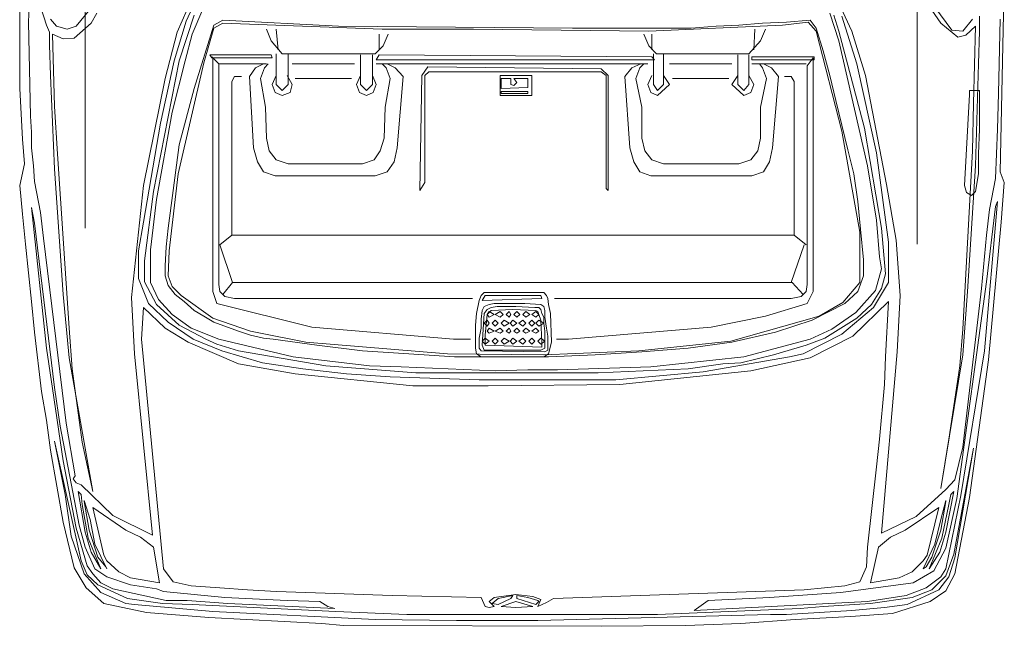
# Model space of a CAD drawing. Units: inches. Extents: x -9 to 646, y -802 to 47.
# Tile 4 of 17: x 432 to 486, y -666 to -633. Entities that reach past the tile are written whole.
import ezdxf

# ---------------------------------------------------------------- set-up
doc = ezdxf.new("R2010")
doc.units = ezdxf.units.IN
doc.header["$MEASUREMENT"] = 0
doc.layers.add('A-SITE-VEHI', color=8, linetype='Continuous', lineweight=9)

msp = doc.modelspace()

# ---------------------------------------------------------------- linework, layer by layer
at = {"layer": 'A-SITE-VEHI'}
for p, q in [((435.913, -624.106), (435.913, -643.944)), ((481.443, -624.866), (481.443, -644.812)), ((432.336, -626.818), (432.336, -636.303)), ((432.933, -629.311), (432.824, -632.671)), ((485.995, -640.855), (486.213, -630.124)), ((433.799, -632.833), (433.311, -631.316)), ((440.953, -633.212), (441.93, -630.99)), ((442.092, -631.207), (441.442, -632.617)), ((477.864, -633.159), (476.836, -630.936)), ((436.184, -631.967), (435.425, -632.888)), ((442.363, -631.967), (441.766, -633.321)), ((483.339, -633.104), (482.418, -631.858)), ((434.341, -632.888), (434.017, -632.509)), ((436.564, -632.182), (436.239, -632.726)), ((441.875, -632.291), (441.062, -634.785)), ((477.16, -633.701), (476.672, -632.182)), ((477.16, -633.159), (476.889, -632.291)), ((478.137, -634.947), (477.322, -632.346)), ((482.256, -632.02), (482.742, -632.726)), ((484.479, -632.509), (483.935, -633.159)), ((484.856, -633.159), (484.856, -632.346)), ((485.995, -632.509), (485.886, -636.574)), ((432.824, -632.671), (432.933, -637.82)), ((433.961, -633.212), (433.799, -632.833)), ((434.938, -633.05), (434.341, -632.888)), ((435.425, -632.888), (434.938, -633.05)), ((436.239, -632.726), (435.318, -633.539)), ((441.442, -632.617), (440.791, -634.785)), ((442.958, -632.833), (441.875, -636.303)), ((442.958, -632.997), (442.417, -634.893)), ((443.447, -632.562), (442.958, -632.833)), ((443.447, -632.726), (442.958, -632.997)), ((449.789, -632.888), (443.447, -632.562)), ((452.173, -633.05), (443.447, -632.726)), ((445.832, -633.05), (446.103, -633.701)), ((446.374, -633.05), (446.482, -634.189)), ((462.581, -632.997), (449.789, -632.888)), ((457.16, -633.05), (452.173, -633.05)), ((466.753, -633.159), (457.16, -633.05)), ((469.084, -632.997), (462.581, -632.997)), ((474.071, -632.833), (466.753, -633.159)), ((470.439, -632.888), (469.084, -632.997)), ((471.687, -632.833), (470.439, -632.888)), ((472.988, -632.726), (471.687, -632.833)), ((472.553, -633.05), (472.499, -634.189)), ((473.15, -633.05), (472.879, -633.701)), ((474.287, -632.671), (472.988, -632.726)), ((475.479, -632.671), (474.071, -632.833)), ((475.588, -632.562), (474.287, -632.671)), ((475.914, -633.159), (475.479, -632.671)), ((475.914, -632.997), (475.588, -632.562)), ((476.294, -634.243), (475.914, -632.997)), ((482.742, -632.726), (483.664, -633.483)), ((484.099, -633.377), (484.641, -632.888)), ((484.641, -632.888), (484.532, -637.116)), ((433.961, -633.919), (433.961, -633.212)), ((434.721, -633.592), (434.125, -633.321)), ((434.125, -633.321), (434.232, -637.278)), ((435.318, -633.539), (434.721, -633.592)), ((440.303, -635.761), (440.953, -633.212)), ((441.766, -633.321), (441.389, -634.785)), ((452.011, -633.321), (452.011, -634.189)), ((452.229, -633.972), (452.5, -633.321)), ((466.753, -633.972), (466.482, -633.321)), ((466.917, -633.321), (466.917, -634.189)), ((477.322, -638.633), (475.914, -633.159)), ((478.57, -638.47), (477.16, -633.159)), ((478.623, -635.597), (477.864, -633.159)), ((483.935, -633.159), (483.339, -633.104)), ((483.664, -633.483), (484.099, -633.377)), ((484.803, -634.947), (484.856, -633.159)), ((434.017, -635.597), (433.961, -633.919)), ((446.103, -633.701), (446.7, -634.405)), ((451.794, -634.405), (452.229, -633.972)), ((467.188, -634.405), (466.753, -633.972)), ((472.879, -633.701), (472.228, -634.405)), ((478.732, -640.531), (477.16, -633.701)), ((446.103, -634.46), (442.743, -634.46)), ((442.743, -634.46), (442.852, -634.622)), ((442.852, -634.569), (443.232, -634.947)), ((442.852, -634.622), (446.158, -634.622)), ((442.905, -634.622), (442.905, -647.414)), ((446.158, -634.622), (446.103, -634.46)), ((446.374, -636.086), (446.374, -634.405)), ((446.7, -634.405), (451.794, -634.405)), ((447.024, -634.405), (447.024, -636.086)), ((450.981, -636.086), (450.981, -634.46)), ((451.632, -634.46), (451.632, -636.086)), ((452.011, -634.46), (451.849, -634.731)), ((466.917, -634.569), (452.011, -634.46)), ((467.079, -634.731), (466.917, -634.569)), ((467.024, -636.086), (467.024, -634.405)), ((472.228, -634.405), (467.188, -634.405)), ((467.568, -634.405), (467.568, -636.086)), ((471.631, -636.086), (471.631, -634.46)), ((472.228, -634.46), (472.228, -636.086)), ((475.806, -634.569), (472.39, -634.569)), ((472.39, -634.569), (472.39, -634.731)), ((475.752, -634.622), (475.426, -635.055)), ((475.752, -634.622), (475.752, -647.414)), ((475.806, -634.731), (475.806, -634.569)), ((476.672, -635.597), (476.294, -634.243)), ((441.062, -634.785), (439.652, -641.939)), ((440.791, -634.785), (440.032, -638.2)), ((441.389, -634.785), (440.683, -637.602)), ((442.417, -634.893), (441.009, -640.964)), ((445.832, -634.947), (443.232, -634.947)), ((443.232, -634.947), (443.232, -647.035)), ((444.91, -635.653), (445.237, -635.164)), ((445.237, -635.164), (445.67, -634.947)), ((445.507, -635.761), (445.723, -635.164)), ((445.723, -635.164), (445.941, -634.947)), ((450.657, -634.947), (447.242, -634.947)), ((451.849, -634.731), (467.079, -634.731)), ((466.699, -634.947), (451.849, -634.947)), ((452.173, -634.947), (452.391, -635.164)), ((452.391, -635.164), (452.606, -635.761)), ((452.444, -634.947), (452.877, -635.164)), ((452.877, -635.164), (453.312, -635.653)), ((454.667, -635.111), (454.343, -635.597)), ((464.153, -635.218), (454.667, -635.111)), ((465.454, -635.653), (465.831, -635.164)), ((465.831, -635.164), (466.32, -634.947)), ((466.049, -635.761), (466.266, -635.164)), ((466.266, -635.164), (466.482, -634.947)), ((471.307, -634.947), (467.892, -634.947)), ((472.39, -634.731), (475.806, -634.731)), ((475.372, -634.947), (472.39, -634.947)), ((472.823, -634.947), (472.988, -635.164)), ((472.988, -635.164), (473.203, -635.761)), ((473.041, -634.947), (473.474, -635.164)), ((473.474, -635.164), (473.854, -635.653)), ((475.426, -635.055), (475.426, -647.035)), ((479.221, -639.825), (478.137, -634.947)), ((484.641, -640.531), (484.803, -634.947)), ((434.232, -640.693), (434.017, -635.597)), ((444.098, -635.653), (443.935, -635.924)), ((444.477, -635.653), (444.098, -635.653)), ((445.128, -639.554), (444.91, -635.653)), ((446.158, -636.086), (446.374, -635.597)), ((446.971, -635.597), (447.242, -636.086)), ((450.763, -636.086), (450.981, -635.597)), ((451.632, -635.597), (451.849, -636.086)), ((453.312, -635.653), (452.986, -639.554)), ((454.343, -635.597), (454.234, -641.886)), ((454.505, -635.597), (454.72, -635.382)), ((454.505, -641.452), (454.505, -635.597)), ((454.72, -635.382), (464.153, -635.382)), ((460.358, -635.597), (458.624, -635.597)), ((458.624, -635.597), (458.624, -636.683)), ((460.358, -636.683), (460.358, -635.597)), ((464.532, -635.597), (464.153, -635.218)), ((464.153, -635.382), (464.423, -635.597)), ((464.423, -635.597), (464.423, -641.777)), ((464.532, -641.886), (464.532, -635.597)), ((465.725, -639.554), (465.454, -635.653)), ((466.699, -636.086), (466.917, -635.597)), ((467.568, -635.597), (467.892, -636.086)), ((471.307, -636.086), (471.631, -635.597)), ((472.228, -635.597), (472.499, -636.086)), ((473.854, -635.653), (473.53, -639.554)), ((474.18, -635.653), (474.558, -635.653)), ((474.558, -635.653), (474.722, -635.924)), ((476.998, -636.954), (476.672, -635.597)), ((479.762, -641.559), (478.623, -635.597)), ((439.11, -641.615), (440.303, -635.761)), ((443.935, -635.924), (443.935, -644.324)), ((445.778, -637.331), (445.507, -635.761)), ((446.32, -636.519), (446.158, -636.086)), ((446.7, -636.41), (446.374, -636.086)), ((447.024, -636.086), (446.7, -636.41)), ((447.242, -636.086), (447.133, -636.519)), ((447.404, -635.761), (450.492, -635.761)), ((450.928, -636.519), (450.763, -636.086)), ((451.307, -636.41), (450.981, -636.086)), ((451.632, -636.086), (451.307, -636.41)), ((451.849, -636.086), (451.685, -636.519)), ((452.606, -635.761), (452.335, -637.331)), ((459.219, -635.761), (458.677, -635.761)), ((458.677, -635.761), (458.677, -636.303)), ((458.677, -636.303), (460.14, -636.248)), ((459.219, -636.086), (459.219, -635.761)), ((459.383, -636.139), (459.219, -636.086)), ((460.14, -635.761), (459.383, -635.761)), ((459.383, -635.761), (459.545, -635.977)), ((459.545, -635.977), (459.383, -636.139)), ((460.14, -636.248), (460.14, -635.761)), ((466.375, -637.331), (466.049, -635.761)), ((466.862, -636.519), (466.699, -636.086)), ((467.241, -636.41), (467.024, -636.086)), ((467.892, -636.086), (467.241, -636.683)), ((467.568, -636.086), (467.241, -636.41)), ((468.054, -635.761), (471.145, -635.761)), ((471.957, -636.683), (471.307, -636.086)), ((471.957, -636.41), (471.631, -636.086)), ((472.228, -636.086), (471.957, -636.41)), ((472.499, -636.086), (472.337, -636.519)), ((473.203, -635.761), (472.879, -637.331)), ((474.722, -635.924), (474.722, -644.324)), ((432.336, -636.303), (432.498, -639.068)), ((441.875, -636.303), (441.062, -639.392)), ((446.7, -636.683), (446.32, -636.519)), ((447.133, -636.519), (446.7, -636.683)), ((451.307, -636.683), (450.928, -636.519)), ((451.685, -636.519), (451.307, -636.683)), ((458.624, -636.683), (460.358, -636.683)), ((460.14, -636.465), (458.677, -636.465)), ((458.677, -636.465), (458.677, -636.574)), ((458.677, -636.574), (460.14, -636.574)), ((460.14, -636.574), (460.14, -636.465)), ((467.241, -636.683), (466.862, -636.519)), ((472.337, -636.519), (471.957, -636.683)), ((484.314, -636.628), (484.043, -641.615)), ((484.856, -636.41), (484.314, -636.41)), ((484.314, -636.41), (484.314, -636.628)), ((484.856, -638.524), (484.856, -636.41)), ((485.886, -636.574), (485.833, -638.524)), ((434.232, -637.278), (434.396, -639.88)), ((445.832, -639.012), (445.778, -637.331)), ((452.335, -637.331), (452.282, -639.012)), ((466.375, -639.012), (466.375, -637.331)), ((472.879, -637.331), (472.879, -639.012)), ((477.322, -638.308), (476.998, -636.954)), ((484.532, -637.116), (484.479, -639.716)), ((432.933, -637.82), (432.986, -638.688)), ((440.683, -637.602), (439.816, -642.374)), ((440.032, -638.2), (439.11, -643.62)), ((477.648, -639.663), (477.322, -638.308)), ((432.986, -638.688), (432.986, -639.554)), ((478.299, -644.161), (477.322, -638.633)), ((479.491, -643.944), (478.57, -638.47)), ((484.803, -639.88), (484.856, -638.524)), ((485.833, -638.524), (485.724, -641.235)), ((432.498, -639.068), (432.607, -640.422)), ((441.062, -639.392), (440.738, -641.886)), ((445.994, -639.716), (445.832, -639.012)), ((452.282, -639.012), (452.065, -639.716)), ((466.537, -639.716), (466.375, -639.012)), ((472.879, -639.012), (472.717, -639.716)), ((432.986, -639.554), (433.095, -640.531)), ((434.396, -639.88), (435.047, -649.419)), ((445.343, -640.313), (445.128, -639.554)), ((446.374, -640.205), (445.994, -639.716)), ((452.065, -639.716), (451.74, -640.205)), ((452.986, -639.554), (452.824, -640.313)), ((465.94, -640.313), (465.725, -639.554)), ((466.917, -640.205), (466.537, -639.716)), ((472.717, -639.716), (472.337, -640.205)), ((473.53, -639.554), (473.365, -640.313)), ((477.973, -640.964), (477.648, -639.663)), ((479.871, -644.703), (479.221, -639.825)), ((484.479, -639.716), (483.935, -649.473)), ((484.803, -640.964), (484.803, -639.88)), ((432.607, -640.422), (432.336, -641.615)), ((433.095, -640.531), (433.149, -641.397)), ((445.67, -640.855), (445.343, -640.313)), ((447.024, -640.422), (446.374, -640.205)), ((451.09, -640.422), (447.024, -640.422)), ((451.74, -640.205), (451.09, -640.422)), ((452.824, -640.313), (452.444, -640.855)), ((466.266, -640.855), (465.94, -640.313)), ((467.568, -640.422), (466.917, -640.205)), ((471.687, -640.422), (467.568, -640.422)), ((472.337, -640.205), (471.687, -640.422)), ((473.365, -640.313), (473.041, -640.855)), ((479.221, -643.511), (478.732, -640.531)), ((484.206, -647.414), (484.641, -640.531)), ((434.721, -647.577), (434.232, -640.693)), ((441.009, -640.964), (440.52, -645.192)), ((446.32, -641.073), (445.67, -640.855)), ((451.794, -641.073), (446.32, -641.073)), ((452.444, -640.855), (451.794, -641.073)), ((466.862, -641.073), (466.266, -640.855)), ((472.39, -641.073), (466.862, -641.073)), ((473.041, -640.855), (472.39, -641.073)), ((478.19, -642.481), (477.973, -640.964)), ((484.641, -641.939), (484.803, -640.964)), ((486.213, -641.452), (485.995, -640.855)), ((432.336, -641.615), (432.498, -643.187)), ((433.149, -641.397), (433.475, -643.078)), ((438.46, -647.739), (439.11, -641.615)), ((454.234, -641.886), (454.505, -641.452)), ((480.304, -644.594), (479.762, -641.559)), ((484.043, -641.615), (484.152, -641.994)), ((485.724, -641.235), (485.398, -642.916)), ((486.048, -643.62), (486.213, -641.452)), ((439.652, -641.939), (439.166, -645.734)), ((440.738, -641.886), (440.467, -643.944)), ((464.423, -641.777), (464.532, -641.886)), ((484.152, -641.994), (484.423, -642.156)), ((484.423, -642.156), (484.641, -641.939)), ((439.816, -642.374), (439.49, -645.136)), ((478.352, -643.999), (478.19, -642.481)), ((485.127, -650.665), (485.833, -642.481)), ((485.833, -642.481), (485.724, -642.752)), ((432.498, -643.187), (432.662, -644.812)), ((433.149, -643.673), (432.986, -642.807)), ((432.986, -642.807), (433.799, -650.503)), ((433.475, -643.078), (433.637, -644.488)), ((485.724, -642.752), (485.236, -646.873)), ((485.398, -642.916), (485.236, -644.324)), ((434.232, -652.67), (433.149, -643.673)), ((439.11, -643.62), (438.84, -645.192)), ((479.383, -645.516), (479.221, -643.511)), ((485.345, -651.154), (486.048, -643.62)), ((440.467, -643.944), (440.358, -644.974)), ((443.935, -644.324), (443.285, -644.865)), ((474.722, -644.324), (443.935, -644.324)), ((474.722, -644.324), (475.372, -644.865)), ((478.299, -646.926), (478.299, -644.161)), ((478.514, -645.68), (478.352, -643.999)), ((479.707, -646.437), (479.491, -643.944)), ((485.236, -644.324), (484.965, -647.25)), ((432.662, -644.812), (432.986, -647.956)), ((433.637, -644.488), (434.883, -654.622)), ((443.285, -644.865), (443.989, -646.926)), ((475.264, -644.865), (474.558, -646.926)), ((479.871, -646.926), (479.871, -644.703)), ((480.522, -647.63), (480.304, -644.594)), ((438.84, -645.192), (438.84, -646.708)), ((439.49, -645.136), (439.49, -646.926)), ((440.358, -644.974), (440.303, -646.004)), ((440.52, -645.192), (440.467, -646.546)), ((439.166, -645.734), (439.166, -646.873)), ((478.514, -646.546), (478.514, -645.68)), ((479.491, -646.167), (479.383, -645.516)), ((440.303, -646.004), (440.303, -646.546)), ((479.165, -647.359), (479.491, -646.167)), ((479.491, -647.25), (479.707, -646.437)), ((438.84, -646.708), (439.381, -648.065)), ((439.166, -646.873), (439.816, -648.118)), ((439.49, -646.926), (439.923, -647.847)), ((440.303, -646.546), (440.467, -647.088)), ((440.467, -646.546), (440.683, -647.144)), ((443.232, -647.035), (443.285, -647.414)), ((443.989, -646.926), (443.447, -647.577)), ((474.613, -646.926), (443.989, -646.926)), ((475.208, -647.577), (474.613, -646.926)), ((475.426, -647.035), (475.372, -647.414)), ((477.378, -648.01), (478.299, -646.926)), ((478.19, -647.414), (478.514, -646.546)), ((479.058, -648.28), (479.871, -646.926)), ((485.236, -646.873), (483.61, -658.741)), ((435.047, -651.045), (434.721, -647.577)), ((440.467, -647.088), (440.845, -647.577)), ((440.683, -647.144), (441.171, -647.63)), ((440.845, -647.577), (441.333, -647.956)), ((442.905, -647.414), (443.123, -648.065)), ((443.285, -647.414), (443.556, -647.685)), ((457.756, -647.468), (457.593, -647.63)), ((461.008, -647.468), (457.756, -647.468)), ((461.171, -647.63), (461.008, -647.468)), ((475.372, -647.414), (475.102, -647.685)), ((475.752, -647.414), (475.426, -648.065)), ((477.486, -648.065), (478.19, -647.414)), ((478.081, -648.551), (479.165, -647.359)), ((478.95, -648.118), (479.491, -647.25)), ((484.965, -647.25), (483.935, -655.923)), ((483.935, -650.883), (484.206, -647.414)), ((432.986, -647.956), (433.149, -649.637)), ((438.624, -650.829), (438.46, -647.739)), ((439.381, -648.065), (440.467, -649.093)), ((439.816, -648.118), (441.062, -649.257)), ((439.923, -647.847), (440.683, -648.66)), ((441.171, -647.63), (442.905, -648.878)), ((441.333, -647.956), (441.875, -648.443)), ((443.123, -648.065), (448.325, -649.364)), ((443.556, -647.685), (444.098, -647.794)), ((444.098, -647.794), (457.105, -647.794)), ((457.485, -647.901), (457.323, -648.607)), ((457.593, -647.63), (457.485, -647.901)), ((457.811, -647.63), (457.649, -647.901)), ((457.649, -647.901), (460.9, -647.794)), ((458.026, -648.118), (457.756, -648.227)), ((460.846, -647.63), (457.811, -647.63)), ((458.297, -648.065), (458.026, -648.118)), ((459.978, -648.065), (458.297, -648.065)), ((460.846, -648.118), (459.978, -648.065)), ((460.9, -647.794), (460.846, -647.63)), ((461.008, -648.227), (460.846, -648.118)), ((461.226, -647.794), (461.171, -647.63)), ((461.279, -648.118), (461.226, -647.794)), ((461.388, -648.607), (461.279, -648.118)), ((474.558, -647.794), (461.604, -647.794)), ((475.426, -648.065), (473.15, -648.769)), ((475.102, -647.685), (474.558, -647.794)), ((475.697, -648.986), (477.486, -648.065)), ((476.076, -648.769), (477.378, -648.01)), ((479.871, -647.956), (477.919, -649.852)), ((478.137, -648.878), (478.95, -648.118)), ((479.707, -650.992), (479.871, -647.956)), ((480.357, -650.721), (480.522, -647.63)), ((439.11, -648.28), (439.004, -650.015)), ((440.303, -649.419), (439.11, -648.28)), ((440.683, -648.66), (441.713, -649.419)), ((441.875, -648.443), (442.417, -648.769)), ((457.323, -648.607), (457.269, -649.257)), ((457.649, -648.443), (457.593, -648.931)), ((457.756, -648.227), (457.649, -648.443)), ((457.756, -648.607), (457.649, -650.341)), ((457.92, -648.389), (457.756, -648.607)), ((457.92, -648.66), (457.811, -649.799)), ((458.135, -648.28), (457.92, -648.389)), ((458.135, -648.443), (457.92, -648.66)), ((457.92, -648.66), (458.026, -648.498)), ((458.026, -648.822), (457.92, -648.66)), ((458.026, -648.498), (458.297, -648.66)), ((458.297, -648.66), (458.026, -648.822)), ((458.462, -648.227), (458.135, -648.28)), ((459.328, -648.389), (458.135, -648.443)), ((458.353, -648.66), (458.624, -648.498)), ((458.624, -648.822), (458.353, -648.66)), ((459.492, -648.227), (458.462, -648.227)), ((458.624, -648.498), (458.786, -648.66)), ((458.786, -648.66), (458.624, -648.822)), ((458.948, -648.66), (459.112, -648.498)), ((459.112, -648.822), (458.948, -648.66)), ((459.112, -648.498), (459.219, -648.66)), ((459.219, -648.66), (459.112, -648.822)), ((460.575, -648.443), (459.328, -648.389)), ((459.383, -648.66), (459.545, -648.498)), ((459.545, -648.822), (459.383, -648.66)), ((460.52, -648.28), (459.492, -648.227)), ((459.545, -648.498), (459.707, -648.66)), ((459.707, -648.66), (459.545, -648.822)), ((459.869, -648.66), (460.034, -648.498)), ((460.034, -648.822), (459.869, -648.66)), ((460.034, -648.498), (460.249, -648.66)), ((460.249, -648.66), (460.034, -648.822)), ((460.358, -648.66), (460.575, -648.498)), ((460.575, -648.822), (460.358, -648.66)), ((460.738, -648.28), (460.52, -648.28)), ((460.684, -648.498), (460.575, -648.443)), ((460.575, -648.498), (460.738, -648.66)), ((460.738, -648.66), (460.575, -648.822)), ((460.738, -648.66), (460.684, -648.498)), ((460.846, -648.389), (460.738, -648.28)), ((460.846, -648.986), (460.738, -648.66)), ((460.9, -648.607), (460.846, -648.389)), ((461.008, -648.822), (460.9, -648.607)), ((461.062, -648.443), (461.008, -648.227)), ((461.062, -648.822), (461.062, -648.443)), ((461.441, -650.179), (461.388, -648.607)), ((476.78, -649.473), (478.081, -648.551)), ((477.322, -649.744), (479.058, -648.28)), ((440.467, -649.093), (441.822, -650.015)), ((442.417, -648.769), (442.958, -649.093)), ((442.905, -648.878), (444.966, -649.582)), ((442.958, -649.093), (444.315, -649.582)), ((457.593, -648.931), (457.593, -649.419)), ((457.756, -649.149), (457.92, -648.986)), ((457.92, -649.311), (457.756, -649.149)), ((457.92, -648.986), (458.026, -649.149)), ((458.026, -649.149), (457.92, -649.311)), ((458.191, -649.149), (458.353, -648.986)), ((458.353, -649.311), (458.191, -649.149)), ((458.353, -648.986), (458.515, -649.149)), ((458.515, -649.149), (458.353, -649.311)), ((458.677, -649.149), (458.841, -648.986)), ((458.841, -649.311), (458.677, -649.149)), ((458.841, -648.986), (459.112, -649.149)), ((459.112, -649.149), (458.841, -649.311)), ((459.165, -649.149), (459.328, -648.986)), ((459.328, -649.311), (459.165, -649.149)), ((459.328, -648.986), (459.545, -649.149)), ((459.545, -649.149), (459.328, -649.311)), ((459.654, -649.149), (459.869, -648.986)), ((459.869, -649.311), (459.654, -649.149)), ((459.869, -648.986), (460.034, -649.149)), ((460.034, -649.149), (459.869, -649.311)), ((460.196, -649.149), (460.358, -648.986)), ((460.358, -649.311), (460.196, -649.149)), ((460.358, -648.986), (460.52, -649.149)), ((460.52, -649.149), (460.358, -649.311)), ((460.575, -649.149), (460.738, -648.986)), ((460.738, -649.311), (460.575, -649.149)), ((460.738, -648.986), (461.008, -649.149)), ((461.008, -649.149), (460.738, -649.311)), ((460.9, -650.179), (460.846, -648.986)), ((461.008, -649.149), (461.008, -648.822)), ((461.062, -649.582), (461.008, -649.149)), ((461.171, -649.419), (461.062, -648.822)), ((473.15, -648.769), (470.168, -649.364)), ((471.251, -650.123), (476.076, -648.769)), ((473.692, -649.637), (475.697, -648.986)), ((476.401, -649.961), (478.137, -648.878)), ((433.149, -649.637), (433.528, -652.888)), ((435.047, -649.419), (435.209, -651.642)), ((441.551, -650.179), (440.303, -649.419)), ((441.062, -649.257), (442.525, -650.015)), ((441.713, -649.419), (443.232, -650.015)), ((444.315, -649.582), (444.966, -649.799)), ((444.966, -649.582), (445.507, -649.69)), ((445.507, -649.69), (448.001, -650.179)), ((448.325, -649.364), (456.077, -650.015)), ((457.269, -649.257), (457.269, -650.503)), ((457.593, -649.419), (457.485, -649.961)), ((457.92, -649.582), (458.026, -649.419)), ((458.026, -649.69), (457.92, -649.582)), ((458.026, -649.419), (458.297, -649.582)), ((458.297, -649.582), (458.026, -649.69)), ((458.353, -649.582), (458.624, -649.419)), ((458.624, -649.69), (458.353, -649.582)), ((458.624, -649.419), (458.786, -649.582)), ((458.786, -649.582), (458.624, -649.69)), ((458.948, -649.582), (459.112, -649.419)), ((459.112, -649.69), (458.948, -649.582)), ((459.112, -649.419), (459.219, -649.582)), ((459.219, -649.582), (459.112, -649.69)), ((459.383, -649.582), (459.545, -649.419)), ((459.545, -649.69), (459.383, -649.582)), ((459.545, -649.419), (459.707, -649.582)), ((459.707, -649.582), (459.545, -649.69)), ((459.869, -649.582), (460.034, -649.419)), ((460.034, -649.69), (459.869, -649.582)), ((460.034, -649.419), (460.249, -649.582)), ((460.249, -649.582), (460.034, -649.69)), ((460.358, -649.582), (460.575, -649.419)), ((460.575, -649.69), (460.358, -649.582)), ((460.575, -649.419), (460.738, -649.582)), ((460.738, -649.582), (460.575, -649.69)), ((461.062, -650.503), (461.062, -649.582)), ((461.226, -649.852), (461.171, -649.419)), ((470.168, -649.364), (462.363, -650.015)), ((471.307, -650.179), (473.692, -649.637)), ((475.208, -650.829), (477.322, -649.744)), ((475.588, -650.015), (476.78, -649.473)), ((483.935, -649.473), (483.772, -651.478)), ((439.004, -650.015), (440.196, -662.589)), ((444.315, -651.371), (441.551, -650.179)), ((441.822, -650.015), (443.394, -650.665)), ((442.525, -650.015), (443.123, -650.286)), ((443.123, -650.286), (444.315, -650.665)), ((443.232, -650.015), (447.295, -650.992)), ((444.966, -649.799), (445.67, -649.961)), ((445.67, -649.961), (446.211, -650.015)), ((446.211, -650.015), (448.596, -650.341)), ((448.001, -650.179), (455.75, -650.829)), ((456.077, -650.015), (456.998, -650.015)), ((457.485, -649.961), (457.485, -650.503)), ((457.649, -650.123), (457.811, -649.961)), ((457.811, -650.286), (457.649, -650.123)), ((457.811, -649.799), (457.811, -650.341)), ((457.811, -649.961), (458.026, -650.123)), ((458.026, -650.123), (457.811, -650.286)), ((458.191, -650.123), (458.353, -649.961)), ((458.353, -650.286), (458.191, -650.123)), ((458.353, -649.961), (458.515, -650.123)), ((458.515, -650.123), (458.353, -650.286)), ((458.677, -650.123), (458.841, -649.961)), ((458.841, -650.286), (458.677, -650.123)), ((458.841, -649.961), (459.112, -650.123)), ((459.112, -650.123), (458.841, -650.286)), ((459.165, -650.123), (459.328, -649.961)), ((459.328, -650.286), (459.165, -650.123)), ((459.328, -649.961), (459.545, -650.123)), ((459.545, -650.123), (459.328, -650.286)), ((459.654, -650.123), (459.869, -649.961)), ((459.869, -650.286), (459.654, -650.123)), ((459.869, -649.961), (460.034, -650.123)), ((460.034, -650.123), (459.869, -650.286)), ((460.196, -650.123), (460.358, -649.961)), ((460.358, -650.286), (460.196, -650.123)), ((460.358, -649.961), (460.52, -650.123)), ((460.52, -650.123), (460.358, -650.286)), ((460.684, -650.123), (460.846, -649.961)), ((460.846, -650.286), (460.684, -650.123)), ((460.846, -649.961), (461.062, -650.123)), ((461.062, -650.123), (460.846, -650.286)), ((460.9, -650.45), (460.9, -650.179)), ((461.226, -650.612), (461.226, -649.852)), ((461.279, -650.829), (461.441, -650.179)), ((462.363, -650.015), (461.712, -650.015)), ((466.211, -650.665), (471.251, -650.123)), ((468.922, -650.503), (471.307, -650.179)), ((471.957, -650.992), (475.588, -650.015)), ((475.372, -650.341), (476.401, -649.961)), ((477.919, -649.852), (475.588, -651.045)), ((433.799, -650.503), (434.125, -652.726)), ((439.599, -660.748), (438.624, -650.829)), ((443.394, -650.665), (445.616, -651.316)), ((444.315, -650.665), (449.085, -651.478)), ((448.596, -650.341), (451.09, -650.665)), ((451.09, -650.665), (453.637, -650.829)), ((453.637, -650.829), (456.13, -650.992)), ((455.75, -650.829), (461.008, -650.883)), ((457.269, -650.503), (457.323, -650.829)), ((457.323, -650.829), (457.593, -650.992)), ((457.485, -650.503), (457.593, -650.665)), ((457.593, -650.665), (461.062, -650.721)), ((457.649, -650.341), (457.756, -650.612)), ((457.756, -650.612), (460.846, -650.612)), ((457.811, -650.341), (460.9, -650.45)), ((460.846, -650.612), (461.062, -650.503)), ((461.008, -650.883), (466.211, -650.665)), ((461.008, -650.992), (461.279, -650.829)), ((461.062, -650.721), (461.226, -650.612)), ((463.826, -650.883), (466.375, -650.721)), ((466.375, -650.721), (468.922, -650.503)), ((473.583, -650.883), (475.372, -650.341)), ((474.451, -650.992), (475.208, -650.829)), ((479.491, -660.639), (480.357, -650.721)), ((483.828, -658.579), (485.127, -650.665)), ((436.346, -658.363), (435.047, -651.045)), ((447.404, -651.913), (444.315, -651.371)), ((445.616, -651.316), (447.837, -651.642)), ((447.295, -650.992), (451.469, -651.478)), ((456.13, -650.992), (461.279, -650.992)), ((461.279, -650.992), (463.826, -650.883)), ((466.862, -651.533), (471.957, -650.992)), ((468.922, -651.642), (470.818, -651.371)), ((469.735, -651.804), (474.451, -650.992)), ((470.818, -651.371), (471.795, -651.316)), ((471.795, -651.316), (473.583, -650.883)), ((475.588, -651.045), (472.337, -651.749)), ((479.654, -652.508), (479.707, -650.992)), ((482.742, -658.199), (483.935, -650.883)), ((484.314, -658.688), (485.345, -651.154)), ((435.209, -651.642), (435.751, -655.652)), ((447.837, -651.642), (450.222, -651.913)), ((449.085, -651.478), (454.016, -651.858)), ((451.469, -651.478), (453.204, -651.533)), ((453.204, -651.533), (458.353, -651.749)), ((454.016, -651.858), (463.99, -651.858)), ((458.353, -651.749), (460.14, -651.695)), ((460.14, -651.695), (461.768, -651.695)), ((461.768, -651.695), (466.862, -651.533)), ((463.99, -651.858), (468.922, -651.642)), ((464.965, -652.237), (469.735, -651.804)), ((472.337, -651.749), (465.183, -652.508)), ((483.772, -651.478), (483.177, -655.49)), ((453.854, -652.564), (447.404, -651.913)), ((450.222, -651.913), (452.606, -652.075)), ((452.606, -652.075), (457.485, -652.237)), ((457.485, -652.237), (464.965, -652.237)), ((433.528, -652.888), (433.799, -654.46)), ((434.125, -652.726), (434.721, -656.683)), ((434.558, -654.784), (434.232, -652.67)), ((457.973, -652.564), (453.854, -652.564)), ((465.183, -652.508), (457.973, -652.564)), ((479.383, -655.49), (479.654, -652.508)), ((433.799, -654.46), (434.017, -656.085)), ((435.589, -660.204), (434.558, -654.784)), ((434.883, -654.622), (435.371, -657.495)), ((435.698, -662.156), (434.232, -655.599)), ((434.232, -655.599), (434.829, -658.526)), ((435.751, -655.652), (436.346, -658.363)), ((479.221, -657.007), (479.383, -655.49)), ((483.177, -655.49), (482.742, -658.199)), ((434.017, -656.085), (434.721, -660.042)), ((484.532, -655.977), (483.448, -661.776)), ((483.935, -655.923), (483.502, -657.713)), ((483.502, -661.994), (484.532, -655.977)), ((434.721, -656.683), (435.425, -660.368)), ((478.732, -661.397), (479.221, -657.007)), ((435.371, -657.495), (435.262, -657.657)), ((435.262, -657.657), (435.425, -657.875)), ((483.502, -657.713), (483.013, -658.255)), ((435.425, -657.875), (435.698, -657.984)), ((435.533, -658.363), (435.913, -660.584)), ((435.698, -658.526), (435.533, -658.363)), ((435.698, -657.984), (437.432, -659.662)), ((483.013, -658.255), (481.388, -659.718)), ((483.448, -658.363), (483.013, -660.584)), ((483.284, -658.526), (483.448, -658.363)), ((434.829, -658.526), (435.154, -660.802)), ((435.751, -659.067), (435.698, -658.526)), ((436.184, -659.88), (435.86, -658.85)), ((435.86, -658.85), (435.86, -658.905)), ((435.86, -658.905), (436.131, -660.477)), ((482.742, -659.88), (483.013, -658.85)), ((483.013, -658.905), (482.742, -660.477)), ((483.013, -662.589), (483.828, -658.579)), ((483.61, -658.741), (483.013, -661.452)), ((483.013, -658.85), (483.013, -658.905)), ((483.177, -659.067), (483.284, -658.526)), ((483.502, -662.862), (484.314, -658.688)), ((436.075, -660.91), (435.751, -659.067)), ((438.136, -660.477), (436.346, -659.229)), ((436.346, -659.229), (436.943, -661.832)), ((480.793, -660.477), (482.636, -659.229)), ((482.636, -659.229), (481.985, -661.832)), ((482.798, -660.91), (483.177, -659.067)), ((436.455, -661.235), (436.184, -659.88)), ((437.432, -659.662), (439.599, -660.748)), ((481.388, -659.718), (479.491, -660.639)), ((482.418, -661.235), (482.742, -659.88)), ((434.721, -660.042), (435.318, -662.536)), ((435.425, -660.368), (436.022, -662.427)), ((435.913, -661.397), (435.589, -660.204)), ((436.131, -660.477), (436.617, -661.941)), ((438.948, -660.855), (438.136, -660.477)), ((479.978, -660.855), (480.793, -660.477)), ((482.742, -660.477), (482.256, -661.941)), ((435.154, -660.802), (435.86, -662.862)), ((435.913, -660.584), (436.239, -661.67)), ((436.781, -662.589), (436.075, -660.91)), ((439.652, -661.397), (438.948, -660.855)), ((479.329, -661.397), (479.978, -660.855)), ((482.092, -662.589), (482.798, -660.91)), ((483.013, -660.584), (482.689, -661.67)), ((436.455, -662.589), (435.913, -661.397)), ((437.105, -662.589), (436.455, -661.235)), ((439.979, -663.348), (439.652, -661.397)), ((478.679, -662.482), (478.732, -661.397)), ((478.894, -663.348), (479.329, -661.397)), ((481.767, -662.589), (482.418, -661.235)), ((483.013, -661.452), (482.365, -662.698)), ((436.239, -661.67), (436.781, -662.589)), ((436.617, -661.941), (437.052, -662.482)), ((436.943, -661.832), (437.105, -662.156)), ((481.985, -661.832), (481.767, -662.156)), ((482.256, -661.941), (481.93, -662.482)), ((482.689, -661.67), (482.092, -662.589)), ((483.448, -661.776), (483.013, -662.969)), ((483.177, -663.024), (483.502, -661.994)), ((435.318, -662.536), (435.968, -663.619)), ((436.022, -662.915), (435.698, -662.156)), ((436.022, -662.427), (436.346, -662.862)), ((437.105, -663.024), (436.455, -662.589)), ((437.052, -662.482), (437.105, -662.589)), ((437.105, -662.156), (437.756, -662.753)), ((440.196, -662.589), (440.738, -663.295)), ((478.299, -663.295), (478.679, -662.482)), ((481.767, -662.156), (481.172, -662.753)), ((481.93, -662.482), (481.767, -662.589)), ((482.742, -663.024), (483.013, -662.589)), ((435.86, -662.862), (436.781, -663.89)), ((436.617, -663.457), (436.022, -662.915)), ((436.346, -662.862), (436.781, -663.348)), ((438.407, -663.457), (437.105, -663.024)), ((437.756, -662.753), (438.407, -663.077)), ((438.407, -663.077), (439.979, -663.348)), ((480.466, -663.077), (478.894, -663.348)), ((481.172, -662.753), (480.466, -663.077)), ((482.365, -662.698), (481.226, -663.348)), ((481.93, -663.619), (482.742, -663.024)), ((483.013, -662.969), (482.256, -663.728)), ((482.636, -663.728), (483.177, -663.024)), ((483.013, -663.784), (483.502, -662.862)), ((435.968, -663.619), (436.943, -664.487)), ((438.244, -664.217), (436.617, -663.457)), ((436.781, -663.348), (437.432, -663.675)), ((437.432, -663.675), (440.358, -664.325)), ((439.816, -663.675), (438.407, -663.457)), ((440.196, -663.837), (439.816, -663.675)), ((440.738, -663.295), (441.713, -663.51)), ((441.713, -663.51), (443.285, -663.619)), ((443.285, -663.619), (444.801, -663.728)), ((444.801, -663.728), (446.374, -663.837)), ((461.55, -664.217), (475.264, -663.728)), ((475.264, -663.728), (477.486, -663.51)), ((481.226, -663.348), (477.269, -663.89)), ((477.486, -663.51), (478.299, -663.295)), ((480.846, -664.054), (481.93, -663.619)), ((480.899, -664.541), (482.636, -663.728)), ((482.256, -663.728), (481.172, -664.161)), ((436.781, -663.89), (438.136, -664.487)), ((440.141, -664.487), (438.244, -664.217)), ((443.556, -664.161), (440.196, -663.837)), ((446.971, -664.325), (443.556, -664.161)), ((446.374, -663.837), (448.001, -663.89)), ((448.001, -663.89), (452.715, -664.054)), ((452.715, -664.054), (457.593, -664.161)), ((457.593, -664.161), (457.811, -664.65)), ((458.026, -664.379), (458.297, -664.161)), ((458.515, -664.217), (458.191, -664.487)), ((458.297, -664.161), (459.492, -663.999)), ((459.328, -664.054), (458.515, -664.217)), ((458.515, -664.541), (459.219, -664.217)), ((459.219, -664.217), (459.328, -664.054)), ((459.492, -663.999), (460.411, -664.108)), ((460.14, -664.161), (459.545, -664.054)), ((459.545, -664.054), (459.545, -664.217)), ((459.545, -664.217), (460.575, -664.541)), ((460.684, -664.325), (460.14, -664.161)), ((460.411, -664.108), (460.846, -664.27)), ((460.846, -664.27), (460.684, -664.65)), ((461.171, -664.432), (461.55, -664.217)), ((473.365, -664.161), (470.006, -664.325)), ((477.269, -663.89), (473.365, -664.161)), ((478.732, -664.379), (480.846, -664.054)), ((481.172, -664.161), (478.894, -664.487)), ((482.147, -664.379), (483.013, -663.784)), ((436.943, -664.487), (439.275, -664.976)), ((438.136, -664.487), (438.624, -664.541)), ((438.624, -664.541), (442.905, -664.92)), ((441.766, -664.541), (440.141, -664.487)), ((440.358, -664.325), (441.495, -664.325)), ((441.495, -664.325), (443.718, -664.487)), ((449.626, -664.92), (441.766, -664.541)), ((443.718, -664.487), (449.571, -664.758)), ((448.758, -664.379), (446.971, -664.325)), ((449.193, -664.65), (448.758, -664.379)), ((449.571, -664.758), (449.193, -664.65)), ((457.811, -664.65), (458.026, -664.703)), ((458.297, -664.65), (458.026, -664.379)), ((458.026, -664.703), (458.297, -664.65)), ((458.191, -664.487), (458.515, -664.541)), ((459.492, -664.379), (458.677, -664.65)), ((458.677, -664.65), (459.492, -664.703)), ((460.411, -664.65), (459.492, -664.379)), ((459.492, -664.703), (460.411, -664.65)), ((460.575, -664.541), (460.738, -664.379)), ((460.738, -664.379), (460.684, -664.325)), ((460.684, -664.65), (461.171, -664.432)), ((470.006, -664.325), (469.246, -664.867)), ((469.246, -664.867), (478.732, -664.379)), ((475.046, -664.758), (471.145, -664.92)), ((476.294, -664.65), (475.046, -664.758)), ((478.894, -664.487), (476.294, -664.65)), ((477.864, -664.867), (479.654, -664.703)), ((479.654, -664.703), (480.899, -664.541)), ((480.087, -665.029), (482.147, -664.379)), ((439.275, -664.976), (442.688, -665.247)), ((442.688, -665.247), (448.867, -665.571)), ((442.905, -664.92), (451.794, -665.353)), ((453.528, -665.083), (449.626, -664.92)), ((451.794, -665.353), (456.239, -665.409)), ((467.241, -665.083), (453.528, -665.083)), ((460.684, -665.409), (473.421, -665.083)), ((471.145, -664.92), (467.241, -665.083)), ((471.795, -665.571), (474.775, -665.353)), ((473.421, -665.083), (474.287, -665.083)), ((474.287, -665.083), (477.864, -664.867)), ((474.775, -665.353), (477.811, -665.191)), ((477.811, -665.191), (480.087, -665.029)), ((448.867, -665.571), (450.059, -665.68)), ((450.059, -665.68), (464.153, -665.733)), ((456.239, -665.409), (460.684, -665.409)), ((464.153, -665.733), (468.76, -665.68)), ((468.76, -665.68), (471.795, -665.571))]:
    msp.add_line(p, q, dxfattribs=at)

doc.saveas('drawing.dxf')
